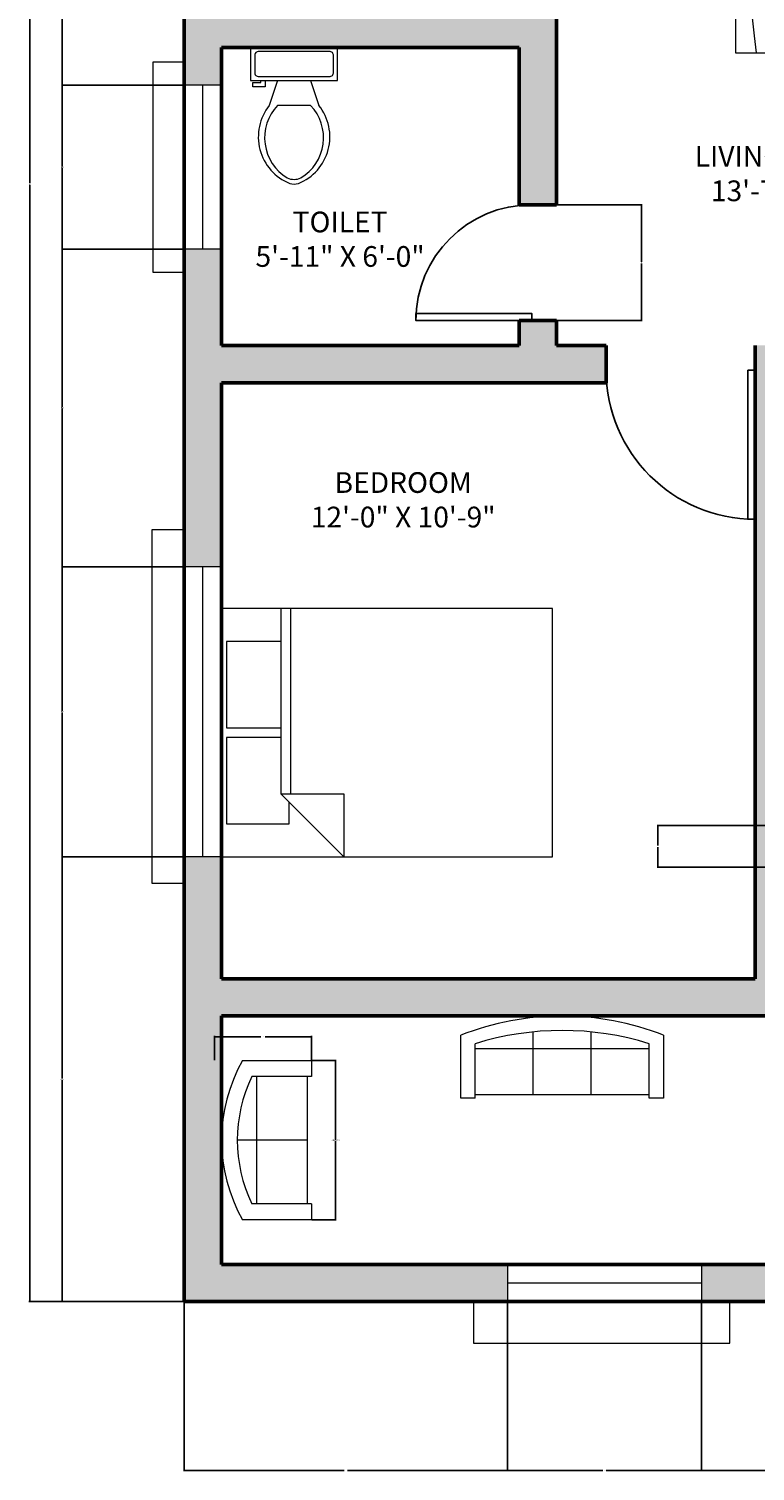
# Model space of a CAD drawing. Units: inches. Extents: x 2710 to 3197, y 524 to 1147.
# Tile 1 of 6: x 2710 to 2885, y 524 to 873. Entities that reach past the tile are written whole.
import ezdxf

# ---------------------------------------------------------------- set-up
doc = ezdxf.new("R2010")
doc.units = ezdxf.units.IN
for name, color, linetype, lineweight in [('A-ANNO-DIMS', 2, 'Continuous', 18), ('A-AREA-IDEN', 7, 'Continuous', 25), ('A-DOOR', 3, 'Continuous', 25), ('A-FLOR-FIXT', 9, 'Continuous', 20), ('A-FURN', 8, 'Continuous', 18), ('A-GLAZ', 4, 'Continuous', 18), ('A-WALL', 7, 'Continuous', 50), ('A-WALL-PATT', 74, 'Continuous', 13)]:
    doc.layers.add(name, color=color, linetype=linetype, lineweight=lineweight)
doc.styles.get("Standard").update_dxf_attribs({"font": 'arial.ttf'})
doc.dimstyles.get("Standard").update_dxf_attribs({"dimtxt": 0.18, "dimasz": 0.18, "dimexe": 0.18, "dimexo": 0.0625, "dimgap": 0.09, "dimtad": 0, "dimtih": 1, "dimtoh": 1, "dimdec": 4, "dimzin": 0, "dimdsep": 46, "dimtxsty": 'Standard', "dimcen": 0.09, "dimadec": 0, "dimazin": 0, "dimtfac": 1, "dimtdec": 4, "dimtofl": 0, "dimtmove": 0, "dimatfit": 3, "dimfxl": 1, "dimtolj": 1, "dimtzin": 0, "dimarcsym": 0})

# ---------------------------------------------------------------- blocks, each defined once
blk = doc.blocks.new('*U9')
for p, q in [((-36, 0), (-36, 6)), ((0, 0), (0, 6))]:
    blk.add_line(p, q)
blk.add_lwpolyline([(0, 0), (0, -36), (-1.75, -36), (-1.75, 0)], close=True)
blk.add_arc((0, 0), 36, 180, 270)
blk = doc.blocks.new('*U6')
for p, q in [((0, 0), (0, -6)), ((28, 0), (28, -6))]:
    blk.add_line(p, q)
blk.add_lwpolyline([(0, 0), (0, 28), (1.75, 28), (1.75, 0)], close=True)
blk.add_arc((0, 0), 28, 0, 90)
blk = doc.blocks.new('Dining Set - 36 x 72 in.')
for p, q in [((-22.2343, 26.00059), (-23.4847, 17.99762)), ((-22.2304, 26), (-5.7608, 26)), ((-22, 27.5), (-22.1562, 26.50042)), ((-5.8416, 26.5), (-22.1534, 26.5)), ((-22, 27.5), (-6, 27.5)), ((-5.8437, 26.49966), (-6, 27.5)), ((-4.5152, 17.99762), (-5.7655, 25.99926)), ((5.7657, 26.00059), (4.5153, 17.99762)), ((5.7696, 26), (22.2392, 26)), ((6, 27.5), (5.8438, 26.50042)), ((22.1584, 26.5), (5.8466, 26.5)), ((6, 27.5), (22, 27.5)), ((22.1563, 26.49966), (22, 27.5)), ((23.4848, 17.99762), (22.2345, 25.99926)), ((36, 18), (-36, 18)), ((-36, 18), (-36, -18)), ((36, -18), (36, 18)), ((-45.5, 8), (-44.5004, 8.15617)), ((-45.5, 8), (-45.5, -8)), ((-44.5, -8.15843), (-44.5, 8.15338)), ((-44.0006, 8.23428), (-35.9976, 9.48474)), ((-44, 8.23041), (-44, -8.23915)), ((44.0006, 8.23428), (35.9976, 9.48474)), ((44, 8.23041), (44, -8.23915)), ((44.5, -8.15843), (44.5, 8.15338)), ((45.5, 8), (44.5005, 8.15617)), ((45.5, 8), (45.5, -8)), ((-44.4997, -8.15631), (-45.5, -8)), ((-35.9976, -9.48476), (-43.9993, -8.2345)), ((35.9976, -9.48476), (43.9993, -8.2345)), ((44.4997, -8.15631), (45.5, -8)), ((-36, -18), (36, -18)), ((-22.2343, -26.0006), (-23.4847, -17.99762)), ((-4.5152, -17.99762), (-5.7655, -25.99928)), ((5.7657, -26.0006), (4.5153, -17.99762)), ((23.4848, -17.99762), (22.2345, -25.99928)), ((-22.2304, -26), (-5.7608, -26)), ((-22, -27.5), (-22.1562, -26.50044)), ((-5.8416, -26.5), (-22.1534, -26.5)), ((-22, -27.5), (-6, -27.5)), ((-5.8437, -26.49967), (-6, -27.5)), ((5.7696, -26), (22.2392, -26)), ((6, -27.5), (5.8438, -26.50044)), ((22.1584, -26.5), (5.8466, -26.5)), ((6, -27.5), (22, -27.5)), ((22.1563, -26.49967), (22, -27.5))]:
    blk.add_line(p, q)
for points in [[(-36, 15), (-31.1772, 14.97754), (-26.8079, 14.91406), (-22.8538, 14.81543), (-19.276, 14.6875), (-16.0362, 14.53613), (-13.0957, 14.36718), (-10.4159, 14.18652), (-7.9583, 14), (-5.6904, 13.81315), (-3.6035, 13.63021), (-1.6954, 13.45508), (0.0365, 13.29166), (1.5945, 13.14388), (2.9811, 13.01562), (4.1988, 12.9108), (5.25, 12.83333), (6.1393, 12.78613), (6.8802, 12.76823), (7.4883, 12.77767), (7.9792, 12.8125), (8.3685, 12.87077), (8.6719, 12.95052), (8.9049, 13.0498), (9.0833, 13.16666), (9.2205, 13.29899), (9.3216, 13.44401), (9.3895, 13.59879), (9.4271, 13.76041), (9.4373, 13.92594), (9.4232, 14.09245), (9.3875, 14.257), (9.3333, 14.41666), (9.2638, 14.56917), (9.1836, 14.71484), (9.0975, 14.85465), (9.0104, 14.98958), (8.9272, 15.1206), (8.8529, 15.2487), (8.7922, 15.37483), (8.75, 15.5), (8.7305, 15.62467), (8.7344, 15.74739), (8.7617, 15.86621), (8.8125, 15.97916), (8.8867, 16.08431), (8.9844, 16.17968), (9.1055, 16.26334), (9.25, 16.33333), (9.4189, 16.38802), (9.6172, 16.42708), (9.8506, 16.45052), (10.125, 16.45833), (10.4463, 16.45052), (10.8203, 16.42708), (11.2529, 16.38802), (11.75, 16.33333), (12.3184, 16.26318), (12.9694, 16.17838), (13.7151, 16.07991), (14.5677, 15.96875), (15.5395, 15.84586), (16.6426, 15.71224), (17.8893, 15.56884), (19.2917, 15.41666), (20.859, 15.25667), (22.5879, 15.08984), (24.4721, 14.91715), (26.5052, 14.73958), (28.6809, 14.5581), (30.9929, 14.3737), (33.4347, 14.18733), (36, 14)], [(-36, 10), (-28.9766, 10.14274), (-23.1725, 10.20442), (-18.4241, 10.19775), (-14.5677, 10.13541), (-11.4399, 10.03011), (-8.877, 9.89453), (-6.7154, 9.74137), (-4.7917, 9.58333), (-2.9698, 9.43082), (-1.2246, 9.28515), (0.4415, 9.14534), (2.026, 9.01041), (3.5266, 8.87939), (4.9408, 8.7513), (6.266, 8.62516), (7.5, 8.5), (8.6411, 8.37549), (9.6914, 8.2539), (10.6538, 8.13818), (11.5312, 8.03125), (12.3267, 7.93603), (13.043, 7.85547), (13.6831, 7.79248), (14.25, 7.75), (14.7471, 7.7303), (15.1797, 7.73307), (15.5537, 7.75732), (15.875, 7.80208), (16.1494, 7.86637), (16.3828, 7.94922), (16.5811, 8.04964), (16.75, 8.16666), (16.8944, 8.29915), (17.0143, 8.44531), (17.1089, 8.60319), (17.1771, 8.77083), (17.218, 8.94629), (17.2305, 9.1276), (17.2137, 9.31282), (17.1667, 9.5), (17.0895, 9.6875), (16.987, 9.875), (16.8649, 10.0625), (16.7292, 10.25), (16.5856, 10.4375), (16.4401, 10.625), (16.2985, 10.8125), (16.1667, 11), (16.05, 11.18733), (15.9518, 11.3737), (15.8752, 11.5581), (15.8229, 11.73958), (15.798, 11.91715), (15.8034, 12.08984), (15.842, 12.25667), (15.9167, 12.41666), (16.0295, 12.56836), (16.1784, 12.70833), (16.3605, 12.83268), (16.5729, 12.9375), (16.8127, 13.01888), (17.0768, 13.07291), (17.3625, 13.0957), (17.6667, 13.08333), (17.9894, 13.03312), (18.3418, 12.94726), (18.7382, 12.82918), (19.1927, 12.68229), (19.7195, 12.51001), (20.3327, 12.31575), (21.0465, 12.10294), (21.875, 11.875), (22.8357, 11.63354), (23.959, 11.37304), (25.2786, 11.08618), (26.8282, 10.76562), (28.6414, 10.40405), (30.752, 9.99414), (33.1936, 9.52856), (36, 9)], [(-36, 5.5), (-30.7157, 5.3348), (-26.069, 5.20963), (-21.9946, 5.11767), (-18.4271, 5.05208), (-15.3009, 5.00602), (-12.5508, 4.97265), (-10.1112, 4.94515), (-7.9167, 4.91666), (-5.909, 4.88167), (-4.0586, 4.83984), (-2.3429, 4.79215), (-0.7396, 4.73958), (0.7739, 4.6831), (2.22, 4.6237), (3.6213, 4.56233), (5, 4.5), (6.373, 4.43782), (7.7344, 4.3776), (9.0723, 4.32129), (10.375, 4.27083), (11.6309, 4.22819), (12.8281, 4.19531), (13.9551, 4.17415), (15, 4.16666), (15.954, 4.17448), (16.819, 4.19791), (17.6001, 4.23698), (18.3021, 4.29166), (18.9299, 4.36198), (19.4883, 4.44791), (19.9823, 4.54948), (20.4167, 4.66666), (20.7969, 4.79899), (21.1302, 4.94401), (21.4245, 5.09879), (21.6875, 5.26041), (21.9271, 5.42594), (22.1511, 5.59245), (22.3672, 5.757), (22.5834, 5.91666), (22.8065, 6.06868), (23.0404, 6.21093), (23.2879, 6.34147), (23.5521, 6.45833), (23.8358, 6.55957), (24.142, 6.64323), (24.4735, 6.70735), (24.8334, 6.75), (25.2235, 6.76969), (25.642, 6.76692), (26.0858, 6.74267), (26.5521, 6.69791), (27.0379, 6.63362), (27.5404, 6.55078), (28.0565, 6.45036), (28.5834, 6.33333), (29.1242, 6.19987), (29.7071, 6.04687), (30.3661, 5.87044), (31.1354, 5.66666), (32.0493, 5.43164), (33.142, 5.16146), (34.4475, 4.85221), (36, 4.5)], [(-36, -1), (-30.7915, -0.6591), (-26.0195, -0.38216), (-21.6519, -0.16284), (-17.6563, 0.00521), (-14.0005, 0.12833), (-10.6523, 0.21289), (-7.5796, 0.26522), (-4.75, 0.29166), (-2.134, 0.29793), (0.2878, 0.28711), (2.5317, 0.26163), (4.6146, 0.22396), (6.5529, 0.17651), (8.3633, 0.12174), (10.0623, 0.06209), (11.6667, 0), (13.1899, -0.06201), (14.6341, -0.1211), (15.9982, -0.17432), (17.2813, -0.21875), (18.4823, -0.25147), (19.6003, -0.26953), (20.6343, -0.27002), (21.5834, -0.25), (22.4481, -0.20768), (23.2357, -0.14584), (23.9549, -0.06836), (24.6146, 0.02083), (25.2235, 0.11784), (25.7904, 0.21875), (26.3241, 0.31966), (26.8334, 0.41666), (27.3265, 0.50618), (27.8099, 0.58593), (28.2894, 0.65397), (28.7709, 0.70833), (29.2601, 0.74707), (29.763, 0.76823), (30.2855, 0.76985), (30.8334, 0.75), (31.4088, 0.70784), (31.9994, 0.64713), (32.589, 0.57275), (33.1615, 0.48958), (33.7008, 0.4025), (34.1908, 0.3164), (34.6153, 0.23616), (34.9584, 0.16666), (35.2099, 0.11165), (35.3848, 0.07031), (35.504, 0.04069), (35.5886, 0.02083), (35.6594, 0.00879), (35.7377, 0.0026), (35.8442, 0.00032), (36, 0)], [(-36, -6.5), (-27.1843, -6.31267), (-20.084, -6.1263), (-14.469, -5.9419), (-10.1094, -5.76042), (-6.7752, -5.58285), (-4.2363, -5.41016), (-2.2629, -5.24333), (-0.625, -5.08334), (0.8708, -4.93099), (2.2715, -4.78646), (3.5872, -4.64974), (4.8281, -4.52084), (6.0046, -4.39974), (7.127, -4.28646), (8.2053, -4.18099), (9.25, -4.08334), (10.2705, -3.99382), (11.2734, -3.91407), (12.2647, -3.84603), (13.25, -3.79167), (14.2354, -3.75293), (15.2266, -3.73177), (16.2295, -3.73015), (17.25, -3.75), (18.2912, -3.79248), (19.3451, -3.85547), (20.4009, -3.93604), (21.4479, -4.03125), (22.4754, -4.13819), (23.4727, -4.25391), (24.4289, -4.37549), (25.3334, -4.5), (26.1785, -4.62492), (26.9694, -4.74935), (27.7145, -4.87281), (28.4219, -4.99479), (29.1, -5.11483), (29.7572, -5.23242), (30.4016, -5.34709), (31.0417, -5.45834), (31.6837, -5.56437), (32.3262, -5.65821), (32.9658, -5.73153), (33.599, -5.77604), (34.2224, -5.78345), (34.8327, -5.74545), (35.4264, -5.65373), (36, -5.5)], [(-36, -10), (-26.4022, -9.81299), (-18.4675, -9.62891), (-11.9839, -9.45069), (-6.7396, -9.28125), (-2.5226, -9.12354), (0.8789, -8.98047), (3.6769, -8.85498), (6.0833, -8.75), (8.2767, -8.66765), (10.3021, -8.60677), (12.1712, -8.56543), (13.8958, -8.54167), (15.4876, -8.53353), (16.9583, -8.53907), (18.3197, -8.55632), (19.5834, -8.58334), (20.7616, -8.61841), (21.8685, -8.66081), (22.9188, -8.71004), (23.9271, -8.76563), (24.9081, -8.82707), (25.8763, -8.89388), (26.8465, -8.96558), (27.8334, -9.04167), (28.8474, -9.12118), (29.8828, -9.20117), (30.93, -9.27824), (31.9792, -9.34896), (33.0205, -9.40991), (34.0443, -9.45768), (35.0407, -9.48885), (36, -9.5)], [(-36, -14.5), (-30.0881, -14.33513), (-25.0332, -14.21224), (-20.7312, -14.12647), (-17.0781, -14.07292), (-13.97, -14.04671), (-11.3027, -14.04297), (-8.9724, -14.05681), (-6.875, -14.08334), (-4.9224, -14.11833), (-3.0905, -14.16016), (-1.3709, -14.20785), (0.2448, -14.26042), (1.7647, -14.3169), (3.1973, -14.3763), (4.5507, -14.43767), (5.8333, -14.5), (7.0554, -14.5621), (8.235, -14.62175), (9.3922, -14.67652), (10.5469, -14.72396), (11.7192, -14.76164), (12.929, -14.78711), (14.1965, -14.79794), (15.5417, -14.79167), (16.9933, -14.76424), (18.6152, -14.70508), (20.4804, -14.60197), (22.6615, -14.44271), (25.2312, -14.21509), (28.2624, -13.9069), (31.8277, -13.50594), (36, -13)]]:
    blk.add_lwpolyline(points)
blk = doc.blocks.new('Sofa - Roundback 7 ft.')
for p, q in [((-36.000027, -34), (-36.000027, -11.4696)), ((-12.00002, -32.4421), (-12.00003, -6.5971)), ((11.99997, -32.4421), (11.99998, -6.5971)), ((35.99998, -34), (35.99998, -11.4696)), ((-35.999844, -13.3819), (35.9998, -13.3819)), ((-36.000027, -32.4421), (35.99998, -32.4421))]:
    blk.add_line(p, q)
for points in [[(-36.000027, -34), (-42.000027, -34), (-42.000027, -8)], [(41.99998, -8), (41.99998, -34), (35.99998, -34)]]:
    blk.add_lwpolyline(points)
for centre, radius, start, end in [((0, -114.25), 114.25, 68.43141, 111.5686), ((-0.00001, -127.1968), 121.1968, 72.72033, 107.2797)]:
    blk.add_arc(centre, radius, start, end)
blk = doc.blocks.new('Sofa - Roundback Loveseat 5 ft.')
for p, q in [((0, -32.44198), (0, -5.99998)), ((-24, -33.99998), (-24, -11.46958)), ((-23.9998, -13.38178), (23.99986, -13.38178)), ((24.00004, -33.99998), (24.00004, -11.46958)), ((-24, -32.44198), (24.00004, -32.44198))]:
    blk.add_line(p, q)
for points in [[(-24, -33.99998), (-30, -33.99998), (-30, -7.99998)], [(30.00004, -7.99998), (30.00004, -33.99998), (24.00004, -33.99998)]]:
    blk.add_lwpolyline(points)
for centre, radius, start, end in [((0, -60.24998), 60.24998, 60.13715, 119.8628), ((0, -61.38438), 55.38444, 64.32083, 115.6792)]:
    blk.add_arc(centre, radius, start, end)
blk = doc.blocks.new('Bed - Queen')
for p, q in [((0, -80.00003), (0, 0)), ((0, 0), (59.99999, 0)), ((59.99999, 0), (59.99999, -80.00003)), ((7.99999, -1.2), (28.79998, -1.2)), ((7.99999, -14.4), (7.99999, -1.2)), ((28.79998, -1.2), (28.79998, -14.4)), ((31.19999, -1.2), (51.99999, -1.2)), ((31.19999, -14.4), (31.19999, -1.2)), ((51.99999, -1.2), (51.99999, -16.4)), ((0, -14.4), (44.8, -14.4)), ((44.8, -16.8), (0, -16.8)), ((59.99999, -29.6), (44.8, -14.4)), ((44.8, -14.4), (44.8, -29.6)), ((51.99999, -16.4), (46.79936, -16.4)), ((44.8, -29.6), (59.99999, -29.6)), ((59.99999, -80.00003), (0, -80.00003))]:
    blk.add_line(p, q)
blk = doc.blocks.new('Toilet - top')
for p, q in [((9.5, -6), (9.5, -2)), ((-10, -8.5), (-8, -8.5)), ((-10, -9.5), (-10, -8.5)), ((-7, -9.5), (-10, -9.5)), ((-8, -8.5), (-8, -8)), ((-7, -8), (-7, -9.5)), ((-4, -8), (-6, -14)), ((4, -8), (6, -14)), ((4, -14), (-4, -14))]:
    blk.add_line(p, q)
blk.add_lwpolyline([(10.5, -8), (10.5, 0), (-10.5, 0), (-10.5, -8)], close=True)
for points in [[(-9.5, -2), (-9.5, -6)], [(8.5, -1), (-8.5, -1)], [(-8.5, -7), (8.5, -7)]]:
    blk.add_lwpolyline(points)
for centre, radius, start, end in [((-8.62, -1.88), 0.884, 81.8699, 188.1301), ((8.62, -1.88), 0.884, 351.8699, 98.1301), ((-8.62, -6.12), 0.884, 171.8699, 278.1301), ((8.62, -6.12), 0.884, 261.8699, 8.1301), ((3.52, -21.58), 12.17, 141.4691, 247.9714), ((4.2, -21.82), 11.33, 136.3677, 238.9468), ((-3.52, -21.58), 12.17, 292.0284, 38.5307), ((-4.2, -21.82), 11.33, 301.053, 43.6321), ((0, -27.88), 4, 245.7318, 294.2682), ((0, -29), 4, 254.8605, 285.1395)]:
    blk.add_arc(centre, radius, start, end)
blk = doc.blocks.new('*D32')
at = {"layer": 'A-ANNO-DIMS', "color": 0, "lineweight": -2, "transparency": 16777216}
for p, q in [((2778.19, 623.22), (2784.08, 623.22)), ((2783.9, 623.04), (2783.9, 604.18)), ((2783.9, 584.96), (2783.9, 603.82)), ((2778.19, 584.78), (2784.08, 584.78))]:
    blk.add_line(p, q, dxfattribs=at)
at = {"layer": 'A-ANNO-DIMS', "color": 0, "transparency": 16777216}
for points in [[(2783.87, 623.04), (2783.93, 623.04), (2783.9, 623.22)], [(2783.87, 584.96), (2783.93, 584.96), (2783.9, 584.78)]]:
    blk.add_solid(points, dxfattribs=at)
at = {"layer": 'Defpoints', "color": 0, "transparency": 16777216}
for p in [(2778.13, 623.22), (2783.9, 623.22), (2778.13, 584.78)]:
    blk.add_point(p, dxfattribs=at)
at = {"layer": 'A-ANNO-DIMS', "color": 0, "transparency": 16777216, "insert": (2783.9, 604), "char_height": 0.18, "attachment_point": 5}
blk.add_mtext('\\A1;LOVESEAT 38 TYP.', dxfattribs=at)
blk = doc.blocks.new('*D33')
at = {"layer": 'A-ANNO-DIMS', "color": 0, "lineweight": -2, "transparency": 16777216}
for p, q in [((2754.64, 623.29), (2754.64, 629.17)), ((2754.82, 628.99), (2765.86, 628.99)), ((2777.95, 628.99), (2766.92, 628.99)), ((2778.13, 623.29), (2778.13, 629.17))]:
    blk.add_line(p, q, dxfattribs=at)
at = {"layer": 'A-ANNO-DIMS', "color": 0, "transparency": 16777216}
for points in [[(2754.82, 629.02), (2754.82, 628.96), (2754.64, 628.99)], [(2777.95, 629.02), (2777.95, 628.96), (2778.13, 628.99)]]:
    blk.add_solid(points, dxfattribs=at)
at = {"layer": 'Defpoints', "color": 0, "transparency": 16777216}
for p in [(2754.64, 628.99), (2754.64, 623.22), (2778.13, 623.22)]:
    blk.add_point(p, dxfattribs=at)
at = {"layer": 'A-ANNO-DIMS', "color": 0, "transparency": 16777216, "insert": (2766.39, 628.99), "char_height": 0.18, "attachment_point": 5}
blk.add_mtext('\\A1;23 TYP.', dxfattribs=at)
blk = doc.blocks.new('*D35')
at = {"layer": 'A-ANNO-DIMS', "color": 0, "lineweight": -2, "transparency": 16777216}
for p, q in [((2747.29, 1105), (2709.83, 1105)), ((2710.01, 1104.82), (2710.01, 835.18)), ((2710.01, 565.18), (2710.01, 834.82)), ((2747.29, 565), (2709.83, 565))]:
    blk.add_line(p, q, dxfattribs=at)
at = {"layer": 'A-ANNO-DIMS', "color": 0, "transparency": 16777216}
for points in [[(2709.98, 1104.82), (2710.04, 1104.82), (2710.01, 1105)], [(2709.98, 565.18), (2710.04, 565.18), (2710.01, 565)]]:
    blk.add_solid(points, dxfattribs=at)
at = {"layer": 'Defpoints', "color": 0, "transparency": 16777216}
for p in [(2710.01, 1105), (2747.35, 1105), (2747.35, 565)]:
    blk.add_point(p, dxfattribs=at)
at = {"layer": 'A-ANNO-DIMS', "color": 0, "transparency": 16777216, "insert": (2710.01, 835), "char_height": 0.18, "attachment_point": 5}
blk.add_mtext('\\A1;540', dxfattribs=at)
blk = doc.blocks.new('*D43')
at = {"layer": 'A-ANNO-DIMS', "color": 0, "lineweight": -2, "transparency": 16777216}
for p, q in [((2747.35, 564.94), (2747.35, 524.03)), ((2825.51, 564.94), (2825.51, 524.03)), ((2747.53, 524.21), (2786.03, 524.21)), ((2825.33, 524.21), (2786.82, 524.21))]:
    blk.add_line(p, q, dxfattribs=at)
at = {"layer": 'A-ANNO-DIMS', "color": 0, "transparency": 16777216}
for points in [[(2747.53, 524.24), (2747.53, 524.18), (2747.35, 524.21)], [(2825.33, 524.24), (2825.33, 524.18), (2825.51, 524.21)]]:
    blk.add_solid(points, dxfattribs=at)
at = {"layer": 'Defpoints', "color": 0, "transparency": 16777216}
for p in [(2747.35, 565), (2825.51, 565), (2825.51, 524.21)]:
    blk.add_point(p, dxfattribs=at)
at = {"layer": 'A-ANNO-DIMS', "color": 0, "transparency": 16777216, "insert": (2786.43, 524.21), "char_height": 0.18, "attachment_point": 5}
blk.add_mtext('\\A1;78.16', dxfattribs=at)
blk = doc.blocks.new('*D44')
at = {"layer": 'A-ANNO-DIMS', "color": 0, "lineweight": -2, "transparency": 16777216}
for p, q in [((2825.51, 564.94), (2825.51, 524.03)), ((2872.37, 564.94), (2872.37, 524.03)), ((2825.69, 524.21), (2848.54, 524.21)), ((2872.19, 524.21), (2849.34, 524.21))]:
    blk.add_line(p, q, dxfattribs=at)
at = {"layer": 'A-ANNO-DIMS', "color": 0, "transparency": 16777216}
for points in [[(2825.69, 524.24), (2825.69, 524.18), (2825.51, 524.21)], [(2872.19, 524.24), (2872.19, 524.18), (2872.37, 524.21)]]:
    blk.add_solid(points, dxfattribs=at)
at = {"layer": 'Defpoints', "color": 0, "transparency": 16777216}
for p in [(2825.51, 565), (2872.37, 565), (2872.37, 524.21)]:
    blk.add_point(p, dxfattribs=at)
at = {"layer": 'A-ANNO-DIMS', "color": 0, "transparency": 16777216, "insert": (2848.94, 524.21), "char_height": 0.18, "attachment_point": 5}
blk.add_mtext('\\A1;46.87', dxfattribs=at)
blk = doc.blocks.new('*D45')
at = {"layer": 'A-ANNO-DIMS', "color": 0, "lineweight": -2, "transparency": 16777216}
for p, q in [((2872.37, 564.94), (2872.37, 524.03)), ((2924.85, 564.94), (2924.85, 524.03)), ((2872.55, 524.21), (2898.22, 524.21)), ((2924.67, 524.21), (2899, 524.21))]:
    blk.add_line(p, q, dxfattribs=at)
at = {"layer": 'A-ANNO-DIMS', "color": 0, "transparency": 16777216}
for points in [[(2872.55, 524.24), (2872.55, 524.18), (2872.37, 524.21)], [(2924.67, 524.24), (2924.67, 524.18), (2924.85, 524.21)]]:
    blk.add_solid(points, dxfattribs=at)
at = {"layer": 'Defpoints', "color": 0, "transparency": 16777216}
for p in [(2872.37, 565), (2924.85, 565), (2924.85, 524.21)]:
    blk.add_point(p, dxfattribs=at)
at = {"layer": 'A-ANNO-DIMS', "color": 0, "transparency": 16777216, "insert": (2898.61, 524.21), "char_height": 0.18, "attachment_point": 5}
blk.add_mtext('\\A1;52.48', dxfattribs=at)
blk = doc.blocks.new('*D50')
at = {"layer": 'A-ANNO-DIMS', "color": 0, "lineweight": -2, "transparency": 16777216}
for p, q in [((2747.29, 672.45), (2717.67, 672.45)), ((2717.85, 672.27), (2717.85, 618.91)), ((2717.85, 565.18), (2717.85, 618.54)), ((2747.29, 565), (2717.67, 565))]:
    blk.add_line(p, q, dxfattribs=at)
at = {"layer": 'A-ANNO-DIMS', "color": 0, "transparency": 16777216}
for points in [[(2717.82, 672.27), (2717.88, 672.27), (2717.85, 672.45)], [(2717.82, 565.18), (2717.88, 565.18), (2717.85, 565)]]:
    blk.add_solid(points, dxfattribs=at)
at = {"layer": 'Defpoints', "color": 0, "transparency": 16777216}
for p in [(2717.85, 672.45), (2747.35, 672.45), (2747.35, 565)]:
    blk.add_point(p, dxfattribs=at)
at = {"layer": 'A-ANNO-DIMS', "color": 0, "transparency": 16777216, "insert": (2717.85, 618.72), "char_height": 0.18, "attachment_point": 5}
blk.add_mtext('\\A1;107.45', dxfattribs=at)
blk = doc.blocks.new('*D51')
at = {"layer": 'A-ANNO-DIMS', "color": 0, "lineweight": -2, "transparency": 16777216}
for p, q in [((2747.29, 742.56), (2717.67, 742.56)), ((2717.85, 742.38), (2717.85, 707.68)), ((2717.85, 672.63), (2717.85, 707.32)), ((2747.29, 672.45), (2717.67, 672.45))]:
    blk.add_line(p, q, dxfattribs=at)
at = {"layer": 'A-ANNO-DIMS', "color": 0, "transparency": 16777216}
for points in [[(2717.82, 742.38), (2717.88, 742.38), (2717.85, 742.56)], [(2717.82, 672.63), (2717.88, 672.63), (2717.85, 672.45)]]:
    blk.add_solid(points, dxfattribs=at)
at = {"layer": 'Defpoints', "color": 0, "transparency": 16777216}
for p in [(2717.85, 742.56), (2747.35, 742.56), (2747.35, 672.45)]:
    blk.add_point(p, dxfattribs=at)
at = {"layer": 'A-ANNO-DIMS', "color": 0, "transparency": 16777216, "insert": (2717.85, 707.5), "char_height": 0.18, "attachment_point": 5}
blk.add_mtext('\\A1;70.11', dxfattribs=at)
blk = doc.blocks.new('*D52')
at = {"layer": 'A-ANNO-DIMS', "color": 0, "lineweight": -2, "transparency": 16777216}
for p, q in [((2747.29, 819.31), (2717.67, 819.31)), ((2717.85, 819.13), (2717.85, 781.11)), ((2717.85, 742.74), (2717.85, 780.75)), ((2747.29, 742.56), (2717.67, 742.56))]:
    blk.add_line(p, q, dxfattribs=at)
at = {"layer": 'A-ANNO-DIMS', "color": 0, "transparency": 16777216}
for points in [[(2717.82, 819.13), (2717.88, 819.13), (2717.85, 819.31)], [(2717.82, 742.74), (2717.88, 742.74), (2717.85, 742.56)]]:
    blk.add_solid(points, dxfattribs=at)
at = {"layer": 'Defpoints', "color": 0, "transparency": 16777216}
for p in [(2717.85, 819.31), (2747.35, 819.31), (2747.35, 742.56)]:
    blk.add_point(p, dxfattribs=at)
at = {"layer": 'A-ANNO-DIMS', "color": 0, "transparency": 16777216, "insert": (2717.85, 780.93), "char_height": 0.18, "attachment_point": 5}
blk.add_mtext('\\A1;76.75', dxfattribs=at)
blk = doc.blocks.new('*D53')
at = {"layer": 'A-ANNO-DIMS', "color": 0, "lineweight": -2, "transparency": 16777216}
for p, q in [((2747.29, 858.86), (2717.67, 858.86)), ((2717.85, 858.68), (2717.85, 839.26)), ((2717.85, 819.49), (2717.85, 838.9)), ((2747.29, 819.31), (2717.67, 819.31))]:
    blk.add_line(p, q, dxfattribs=at)
at = {"layer": 'A-ANNO-DIMS', "color": 0, "transparency": 16777216}
for points in [[(2717.82, 858.68), (2717.88, 858.68), (2717.85, 858.86)], [(2717.82, 819.49), (2717.88, 819.49), (2717.85, 819.31)]]:
    blk.add_solid(points, dxfattribs=at)
at = {"layer": 'Defpoints', "color": 0, "transparency": 16777216}
for p in [(2717.85, 858.86), (2747.35, 858.86), (2747.35, 819.31)]:
    blk.add_point(p, dxfattribs=at)
at = {"layer": 'A-ANNO-DIMS', "color": 0, "transparency": 16777216, "insert": (2717.85, 839.08), "char_height": 0.18, "attachment_point": 5}
blk.add_mtext('\\A1;39.55', dxfattribs=at)
blk = doc.blocks.new('*D54')
at = {"layer": 'A-ANNO-DIMS', "color": 0, "lineweight": -2, "transparency": 16777216}
for p, q in [((2747.29, 904.83), (2717.67, 904.83)), ((2717.85, 904.65), (2717.85, 882.03)), ((2717.85, 859.04), (2717.85, 881.66)), ((2747.29, 858.86), (2717.67, 858.86))]:
    blk.add_line(p, q, dxfattribs=at)
at = {"layer": 'A-ANNO-DIMS', "color": 0, "transparency": 16777216}
for points in [[(2717.82, 904.65), (2717.88, 904.65), (2717.85, 904.83)], [(2717.82, 859.04), (2717.88, 859.04), (2717.85, 858.86)]]:
    blk.add_solid(points, dxfattribs=at)
at = {"layer": 'Defpoints', "color": 0, "transparency": 16777216}
for p in [(2717.85, 904.83), (2747.35, 904.83), (2747.35, 858.86)]:
    blk.add_point(p, dxfattribs=at)
at = {"layer": 'A-ANNO-DIMS', "color": 0, "transparency": 16777216, "insert": (2717.85, 881.84), "char_height": 0.18, "attachment_point": 5}
blk.add_mtext('\\A1;45.98', dxfattribs=at)
blk = doc.blocks.new('*D75')
at = {"layer": 'A-ANNO-DIMS', "color": 0, "lineweight": -2, "transparency": 16777216}
for p, q in [((2828.41, 830), (2858.03, 830)), ((2857.85, 829.82), (2857.85, 816.18)), ((2857.85, 802.18), (2857.85, 815.82)), ((2828.41, 802), (2858.03, 802))]:
    blk.add_line(p, q, dxfattribs=at)
at = {"layer": 'A-ANNO-DIMS', "color": 0, "transparency": 16777216}
for points in [[(2857.82, 829.82), (2857.88, 829.82), (2857.85, 830)], [(2857.82, 802.18), (2857.88, 802.18), (2857.85, 802)]]:
    blk.add_solid(points, dxfattribs=at)
at = {"layer": 'Defpoints', "color": 0, "transparency": 16777216}
for p in [(2828.35, 830), (2828.35, 802), (2857.85, 802)]:
    blk.add_point(p, dxfattribs=at)
at = {"layer": 'A-ANNO-DIMS', "color": 0, "transparency": 16777216, "insert": (2857.85, 816), "char_height": 0.18, "attachment_point": 5}
blk.add_mtext('\\A1;28', dxfattribs=at)
blk = doc.blocks.new('*D80')
at = {"layer": 'A-ANNO-DIMS', "color": 0, "lineweight": -2, "transparency": 16777216}
for p, q in [((2891.29, 680), (2861.67, 680)), ((2861.85, 679.82), (2861.85, 675.18)), ((2861.85, 670.18), (2861.85, 674.82)), ((2891.29, 670), (2861.67, 670))]:
    blk.add_line(p, q, dxfattribs=at)
at = {"layer": 'A-ANNO-DIMS', "color": 0, "transparency": 16777216}
for points in [[(2861.82, 679.82), (2861.88, 679.82), (2861.85, 680)], [(2861.82, 670.18), (2861.88, 670.18), (2861.85, 670)]]:
    blk.add_solid(points, dxfattribs=at)
at = {"layer": 'Defpoints', "color": 0, "transparency": 16777216}
for p in [(2861.85, 680), (2891.35, 680), (2891.35, 670)]:
    blk.add_point(p, dxfattribs=at)
at = {"layer": 'A-ANNO-DIMS', "color": 0, "transparency": 16777216, "insert": (2861.85, 675), "char_height": 0.18, "attachment_point": 5}
blk.add_mtext('\\A1;10', dxfattribs=at)

msp = doc.modelspace()

# ---------------------------------------------------------------- hatches: boundary and pattern name
at = {"layer": 'A-WALL-PATT'}
h = msp.add_hatch(color=256, dxfattribs=at)
h.dxf.hatch_style = 1
h.paths.add_polyline_path([(2898.3484, 1096.0017), (2898.3484, 967.0017), (2948.3484, 967.0017), (2948.3484, 787.0017), (2957.3484, 787.0017), (2957.3484, 793.0017), (2957.3484, 833.0017), (2957.3484, 967.0017), (3007.3484, 967.0017), (3007.3484, 973.0017), (3007.3484, 1009.0017), (3007.3484, 1096.0017), (3149.3484, 1096.0017), (3149.3484, 1084.4601), (3158.3484, 1084.4601), (3158.3484, 1105.0017), (2991.781, 1105.0017), (2991.781, 1096.0017), (2998.3484, 1096.0017), (2998.3484, 976.0017), (2957.3484, 976.0017), (2957.3484, 1003.0017), (2966.3484, 1003.0017), (2966.3484, 1012.0017), (2957.3484, 1012.0017), (2957.3484, 1096.0017), (2963.4487, 1096.0017), (2963.4487, 1105.0017), (2940.703, 1105.0017), (2940.703, 1096.0017), (2948.3484, 1096.0017), (2948.3484, 1012.0017), (2939.3484, 1012.0017), (2939.3484, 1003.0017), (2948.3484, 1003.0017), (2948.3484, 976.0017), (2907.3484, 976.0017), (2907.3484, 1096.0017), (2916.9598, 1096.0017), (2916.9598, 1105.0017), (2857.03, 1105.0017), (2857.03, 1096.0017)])
h.paths.add_polyline_path([(2789.8274, 1096.0017), (2789.8274, 1105.0017), (2747.3484, 1105.0017), (2747.3484, 943.327), (2756.3484, 943.327), (2756.3484, 967.0017), (2828.3484, 967.0017), (2828.3484, 909.0017), (2837.3484, 909.0017), (2837.3484, 967.0017), (2862.3484, 967.0017), (2862.3484, 973.0017), (2862.3484, 976.0017), (2756.3484, 976.0017), (2756.3484, 1096.0017)])
h.paths.add_polyline_path([(2828.3484, 868.0017), (2828.3484, 830.0017), (2837.3484, 830.0017), (2837.3484, 877.0017), (2756.3484, 877.0017), (2756.3484, 904.8338), (2747.3484, 904.8338), (2747.3484, 858.8554), (2756.3484, 858.8554), (2756.3484, 868.0017)])
h.paths.add_polyline_path([(2747.3484, 742.5572), (2756.3484, 742.5572), (2756.3484, 787.0017), (2849.3484, 787.0017), (2849.3484, 796.0017), (2837.3484, 796.0017), (2837.3484, 802.0017), (2831.3484, 802.0017), (2828.3484, 802.0017), (2828.3484, 796.0017), (2756.3484, 796.0017), (2756.3484, 819.3052), (2747.3484, 819.3052)])
h.paths.add_polyline_path([(2756.3484, 643.0017), (2756.3484, 672.4477), (2747.3484, 672.4477), (2747.3484, 565.0017), (2825.5051, 565.0017), (2825.5051, 574.0017), (2756.3484, 574.0017), (2756.3484, 634.0017), (2891.3484, 634.0017), (2891.3484, 787.0017), (2908.3484, 787.0017), (2908.3484, 793.0017), (2908.3484, 796.0017), (2891.3484, 796.0017), (2885.3484, 796.0017), (2885.3484, 790.0017), (2885.3484, 754.0017), (2885.3484, 643.0017)])
h.paths.add_polyline_path([(2924.8484, 565.0017), (2924.8484, 571.0017), (2924.8484, 574.0017), (2872.3715, 574.0017), (2872.3715, 565.0017)])
h.paths.add_polyline_path([(2984.8484, 574.0017), (2984.8484, 571.0017), (2984.8484, 565.0017), (3050.793, 565.0017), (3050.793, 574.0017)])
h.paths.add_polyline_path([(3158.3484, 565.0017), (3158.3484, 685.5326), (3149.3484, 685.5326), (3149.3484, 675.4542), (3149.3484, 643.0017), (3020.3484, 643.0017), (3020.3484, 796.0017), (3014.3484, 796.0017), (2997.3484, 796.0017), (2997.3484, 787.0017), (3014.3484, 787.0017), (3014.3484, 634.0017), (3149.3484, 634.0017), (3149.3484, 574.0017), (3104.3903, 574.0017), (3104.3903, 565.0017)])
h.paths.add_polyline_path([(3149.3484, 787.0017), (3149.3484, 746.9465), (3158.3484, 746.9465), (3158.3484, 820.3805), (3149.3484, 820.3805), (3149.3484, 796.0017), (3077.3484, 796.0017), (3077.3484, 802.0017), (3074.3484, 802.0017), (3068.3484, 802.0017), (3068.3484, 796.0017), (3056.3484, 796.0017), (3056.3484, 790.0017), (3056.3484, 787.0017)])
h.paths.add_polyline_path([(3158.3484, 905.224), (3149.3484, 905.224), (3149.3484, 877.0017), (3068.3484, 877.0017), (3068.3484, 838.0017), (3074.3484, 838.0017), (3077.3484, 838.0017), (3077.3484, 868.0017), (3149.3484, 868.0017), (3149.3484, 852.3022), (3158.3484, 852.3022)], flags=17)
h.paths.add_polyline_path([(3099.2867, 814.3126), (3142.0289, 814.3126), (3142.0289, 832.97), (3099.2867, 832.97)], flags=25)
h.paths.add_polyline_path([(2981.8144, 832.8032), (3033.605, 832.8032), (3033.605, 851.4605), (2981.8144, 851.4605)], flags=25)

# ---------------------------------------------------------------- linework, layer by layer
at = {"layer": 'A-GLAZ'}
for p, q in [((2747.3484, 864.4118), (2739.7454, 864.4118)), ((2739.7454, 864.4118), (2739.7454, 813.7147)), ((2756.3484, 858.8554), (2747.3484, 858.8554)), ((2751.8484, 819.3052), (2751.8484, 858.8554)), ((2756.3484, 819.3052), (2747.3484, 819.3052)), ((2739.7454, 813.7147), (2747.3484, 813.7147)), ((2747.3484, 751.4698), (2739.5108, 751.4698)), ((2739.5108, 751.4698), (2739.5108, 666.121)), ((2756.3484, 742.5572), (2747.3484, 742.5572)), ((2751.8484, 672.4477), (2751.8484, 742.5572)), ((2756.3484, 672.4477), (2747.3484, 672.4477)), ((2739.5108, 666.121), (2747.3484, 666.121)), ((2825.5051, 574.0017), (2825.5051, 565.0017)), ((2872.3715, 574.0017), (2872.3715, 565.0017)), ((2825.5051, 569.5017), (2872.3715, 569.5017)), ((2817.2429, 565.0017), (2817.2429, 554.9521)), ((2879.2611, 554.9521), (2879.2611, 565.0017)), ((2817.2429, 554.9521), (2879.2611, 554.9521))]:
    msp.add_line(p, q, dxfattribs=at)
at = {"layer": 'A-WALL'}
for p, q in [((2747.3484, 1105.0017), (2747.3484, 565.0017)), ((2837.3484, 877.0017), (2837.3484, 830.0017)), ((2756.3484, 868.0017), (2756.3484, 796.0017)), ((2828.3484, 868.0017), (2756.3484, 868.0017)), ((2828.3484, 868.0017), (2828.3484, 830.0017)), ((2828.3484, 830.0017), (2837.3484, 830.0017)), ((2828.3484, 802.0017), (2837.3484, 802.0017)), ((2828.3484, 802.0017), (2828.3484, 796.0017)), ((2837.3484, 802.0017), (2837.3484, 796.0017)), ((2828.3484, 796.0017), (2756.3484, 796.0017)), ((2849.3484, 796.0017), (2837.3484, 796.0017)), ((2849.3484, 796.0017), (2849.3484, 787.0017)), ((2885.3484, 796.0017), (2885.3484, 643.0017)), ((2756.3484, 787.0017), (2756.3484, 643.0017)), ((2849.3484, 787.0017), (2756.3484, 787.0017)), ((2885.3484, 643.0017), (2756.3484, 643.0017)), ((2756.3484, 634.0017), (2756.3484, 574.0017)), ((2891.3484, 634.0017), (2756.3484, 634.0017)), ((2756.3484, 574.0017), (2924.8484, 574.0017)), ((2747.3484, 565.0017), (2924.8484, 565.0017))]:
    msp.add_line(p, q, dxfattribs=at)

# ---------------------------------------------------------------- block references
at = {"layer": 'A-DOOR', "rotation": 90}
msp.add_blockref('*U6', (2831.3484, 802.0017), dxfattribs=at)
at = {"layer": 'A-DOOR'}
msp.add_blockref('*U9', (2885.3484, 790.0017), dxfattribs=at)
at = {"layer": 'A-FLOR-FIXT'}
msp.add_blockref('Toilet - top', (2773.9163, 868.0017), dxfattribs=at)
at = {"layer": 'A-FURN', "rotation": 270}
msp.add_blockref('Dining Set - 36 x 72 in.', (2898.63, 902.6723), dxfattribs=at)
at = {"layer": 'A-FURN', "xscale": -1, "rotation": 90}
msp.add_blockref('Bed - Queen', (2756.3484, 732.4476), dxfattribs=at)
at = {"layer": 'A-FURN', "xscale": 0.5838396323201516, "yscale": 0.5838396323201516, "zscale": 0.5838396323201516}
msp.add_blockref('Sofa - Roundback 7 ft.', (2838.711, 634.0017), dxfattribs=at)
at = {"layer": 'A-FURN', "xscale": 0.640698906201209, "yscale": 0.640698906201209, "zscale": 0.640698906201209, "rotation": 90}
msp.add_blockref('Sofa - Roundback Loveseat 5 ft.', (2756.3484, 604.0017), dxfattribs=at)

# ---------------------------------------------------------------- texts
at = {"layer": 'A-AREA-IDEN', "char_height": 5, "attachment_point": 1}
for s, insert in [('\\pxqc;LIVING/ DINING\\P13\'-7" X 8\'-4"', (2866.2582, 844.202)), ('\\pxqc;TOILET\\P5\'-11" X 6\'-0"', (2756.2032, 828.3425)), ('\\pxqc;BEDROOM\\P12\'-0" X 10\'-9"', (2771.4541, 765.385))]:
    msp.add_mtext_dynamic_manual_height_columns(s, width=57.655828, gutter_width=12.5, heights=[0], dxfattribs=dict(at, insert=insert))

# ---------------------------------------------------------------- dimensions: what is measured, and where the dimension line sits
at = {"layer": 'A-ANNO-DIMS'}
for base, p1, p2, angle, override, picture, middle in [((2710.0108, 1105.0017), (2747.3484, 565.0017), (2747.3484, 1105.0017), 90, {"dimdec": 0, "dimlfac": 1, "dimrnd": 0, "dimzin": 0, "dimdsep": 46, "dimlunit": 2}, '*D35', (2710.0108, 835.0017)), ((2717.8484, 904.8338), (2747.3484, 858.8554), (2747.3484, 904.8338), 90, {"dimdec": 2, "dimlfac": 1, "dimrnd": 0, "dimzin": 0, "dimdsep": 46, "dimlunit": 2}, '*D54', (2717.8484, 881.8446)), ((2717.8484, 858.8554), (2747.3484, 819.3052), (2747.3484, 858.8554), 90, {"dimdec": 2, "dimlfac": 1, "dimrnd": 0, "dimzin": 0, "dimdsep": 46, "dimlunit": 2}, '*D53', (2717.8484, 839.0803)), ((2857.8484, 802.0017), (2828.3484, 830.0017), (2828.3484, 802.0017), 270, {"dimdec": 0, "dimlfac": 1, "dimrnd": 0, "dimzin": 0, "dimdsep": 46, "dimlunit": 2}, '*D75', (2857.8484, 816.0017)), ((2717.8484, 819.3052), (2747.3484, 742.5572), (2747.3484, 819.3052), 90, {"dimdec": 2, "dimlfac": 1, "dimrnd": 0, "dimzin": 0, "dimdsep": 46, "dimlunit": 2}, '*D52', (2717.8484, 780.9312)), ((2717.8484, 742.5572), (2747.3484, 672.4477), (2747.3484, 742.5572), 90, {"dimdec": 2, "dimlfac": 1, "dimrnd": 0, "dimzin": 0, "dimdsep": 46, "dimlunit": 2}, '*D51', (2717.8484, 707.5024)), ((2861.8484, 680.0017), (2891.3484, 670.0017), (2891.3484, 680.0017), 90, {"dimdec": 0, "dimlfac": 1, "dimrnd": 0, "dimzin": 0, "dimdsep": 46, "dimlunit": 2}, '*D80', (2861.8484, 675.0017)), ((2717.8484, 672.4477), (2747.3484, 565.0017), (2747.3484, 672.4477), 90, {"dimdec": 2, "dimlfac": 1, "dimrnd": 0, "dimzin": 0, "dimdsep": 46, "dimlunit": 2}, '*D50', (2717.8484, 618.7247))]:
    dim = msp.add_linear_dim(base=base, p1=p1, p2=p2, angle=angle, dimstyle='Standard', override=override, dxfattribs=at)
    dim.commit()
    dim.dimension.update_dxf_attribs({"geometry": picture, "text_midpoint": middle})
for base, p1, p2, angle, text, picture, middle in [((2754.6399, 628.9889), (2778.1322, 623.2227), (2754.6399, 623.2227), 180, '<> TYP.', '*D33', (2766.386, 628.9889)), ((2783.8985, 623.2227), (2778.1322, 584.7807), (2778.1322, 623.2227), 90, 'LOVESEAT <> TYP.', '*D32', (2783.8985, 604.0017))]:
    dim = msp.add_linear_dim(base=base, p1=p1, p2=p2, angle=angle, text=text, dimstyle='Standard', override={"dimdec": 0, "dimlfac": 1, "dimrnd": 0, "dimzin": 0, "dimdsep": 46, "dimlunit": 2}, dxfattribs=at)
    dim.commit()
    dim.dimension.update_dxf_attribs({"geometry": picture, "text_midpoint": middle})
for base, p1, p2, picture, middle in [((2825.5051, 524.2139), (2747.3484, 565.0017), (2825.5051, 565.0017), '*D43', (2786.4267, 524.2139)), ((2872.3715, 524.2139), (2825.5051, 565.0017), (2872.3715, 565.0017), '*D44', (2848.9383, 524.2139)), ((2924.8484, 524.2139), (2872.3715, 565.0017), (2924.8484, 565.0017), '*D45', (2898.61, 524.2139))]:
    dim = msp.add_linear_dim(base=base, p1=p1, p2=p2, dimstyle='Standard', override={"dimdec": 2, "dimlfac": 1, "dimrnd": 0, "dimzin": 0, "dimdsep": 46, "dimlunit": 2}, dxfattribs=at)
    dim.commit()
    dim.dimension.update_dxf_attribs({"geometry": picture, "text_midpoint": middle})

doc.saveas('drawing.dxf')
